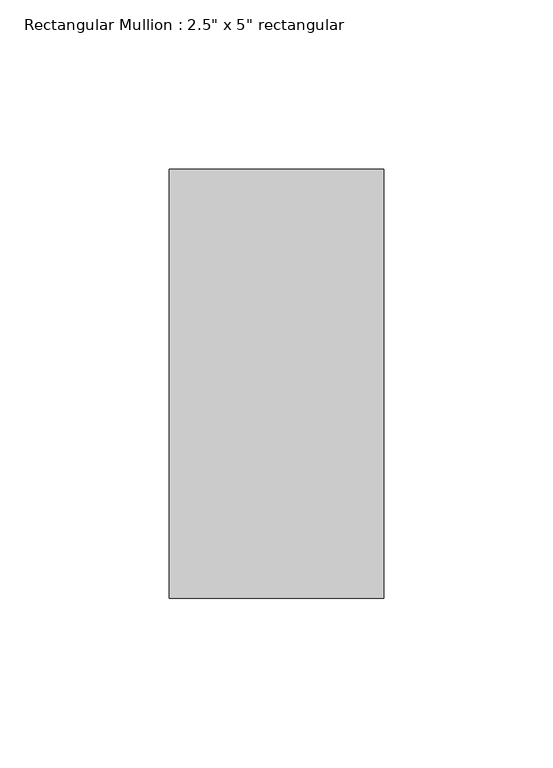
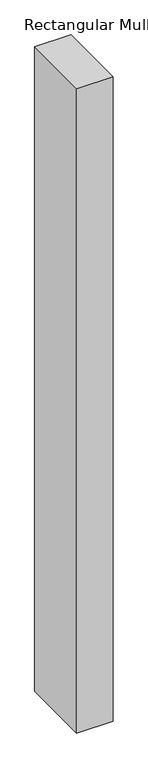
"""IFC4 building model written with IfcOpenShell, lengths in millimetres: member geometry."""

from ifc_helpers import new_model, si_unit, frame, origin, place, context, project, spatial, polyline, outline, extrude, source, transform, mapped, element, save


def member_0e454ba5(model_context):
    return source(origin(), model_context, "Body", "SweptSolid", [
        extrude(outline(polyline([(0.0, 63.5), (0.0, -63.5), (-63.5, -63.5), (-63.5, 63.5), (0.0, 63.5)])), frame((0.0, 0.0, -1187.4500002), z_axis=(0.0, 0.0, 1.0), x_axis=(1.0, 0.0, 0.0)), (0.0, 0.0, 1.0), 1187.4500002),
    ])


if __name__ == "__main__":
    model = new_model("IFC4")
    model_context = context("Model", 3, world=origin())
    ifc_project = project(units=[si_unit("LENGTHUNIT", "METRE", prefix="MILLI")], contexts=[model_context])
    site = spatial("IfcSite", under=ifc_project)
    building = spatial("IfcBuilding", under=site)
    placement = place(None, origin())
    member_shape = member_0e454ba5(model_context)
    element("IfcMember", 1, ObjectType="Rectangular Mullion : 2.5\" x 5\" rectangular", at=placement, inside=building, context=model_context, shape_type="MappedRepresentation", body=[
        mapped(member_shape, transform((0.0, 0.0, 0.0), x_axis=(1.0, 0.0, 0.0), y_axis=(0.0, 1.0, 0.0), z_axis=(0.0, 0.0, 1.0))),
    ])
    save(model, "model.ifc")

# Revit data of these elements
# Type "Rectangular Mullion : 2.5\" x 5\" rectangular"
#   built-in parameter 1007304 = 0.416667 (stored number, unit not read)
#   built-in parameter 1007301 = 0.104167 (stored number, unit not read)
#   built-in parameter 1007300 = 0.104167 (stored number, unit not read)
# Element 1 (IfcMember, "Rectangular Mullion : 2.5\" x 5\" rectangular")
#   Materials on its faces: "Aluminum"
# Materials
#   "Aluminum": class "Metal", colour RGB 247 247 247, transparency 0, Description = "Aluminum 6061", Cost = 0
